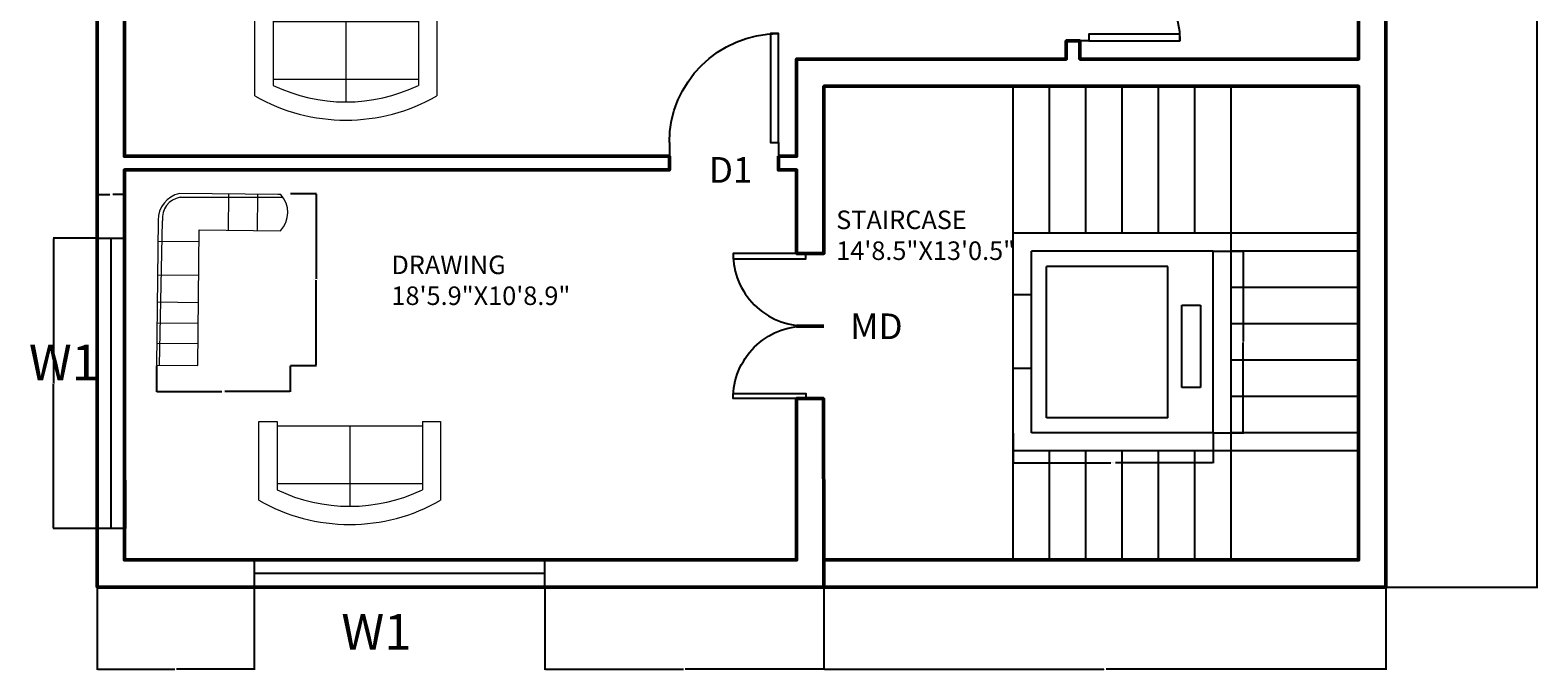
# Model space of a CAD drawing. Units: inches. Extents: x -45 to 1424, y 648 to 1662.
# Tile 5 of 8: x 927 to 1424, y 695 to 906. Entities that reach past the tile are written whole.
import ezdxf

# ---------------------------------------------------------------- set-up
doc = ezdxf.new("R2010")
doc.units = ezdxf.units.IN
for name, color, linetype, lineweight in [('A-ANNO-DIMS', 2, 'Continuous', 18), ('A-ANNO-TEXT', 7, 'Continuous', 18), ('A-AREA-IDEN', 7, 'Continuous', 18), ('A-FLOR-EVTR', 140, 'Continuous', 25), ('DOOR', 2, 'Continuous', 25), ('FURNITURE', 3, 'Continuous', 18), ('STAIRCASE', 140, 'Continuous', 25), ('WALL', 4, 'Continuous', 50), ('WINDOW', 1, 'Continuous', 25)]:
    doc.layers.add(name, color=color, linetype=linetype, lineweight=lineweight)
doc.styles.get("Standard").update_dxf_attribs({"font": 'arial.ttf'})
doc.dimstyles.get("Standard").update_dxf_attribs({"dimtxt": 0.18, "dimasz": 0.18, "dimexe": 0.18, "dimexo": 0.0625, "dimgap": 0.09, "dimtad": 0, "dimtih": 1, "dimtoh": 1, "dimdec": 4, "dimzin": 0, "dimdsep": 46, "dimtxsty": 'Standard', "dimcen": 0.09, "dimadec": 0, "dimazin": 0, "dimtfac": 1, "dimtdec": 4, "dimtofl": 0, "dimtmove": 0, "dimatfit": 3, "dimfxl": 1, "dimtolj": 1, "dimtzin": 0, "dimarcsym": 0})

# ---------------------------------------------------------------- blocks, each defined once
blk = doc.blocks.new('*U5')
for p, q in [((0, 0), (0, -6)), ((24, 0), (24, -6))]:
    blk.add_line(p, q)
blk.add_lwpolyline([(0, 0), (0, 24), (1.75, 24), (1.75, 0)], close=True)
blk.add_arc((0, 0), 24, 0, 90)
blk = doc.blocks.new('*U3')
for p, q in [((0, 0), (0, -6)), ((24, 0), (24, -6))]:
    blk.add_line(p, q)
blk.add_lwpolyline([(0, 0), (0, 24), (1.75, 24), (1.75, 0)], close=True)
blk.add_arc((0, 0), 24, 0, 90)
blk = doc.blocks.new('*U6')
for p, q in [((0, 0), (0, 6)), ((24, 0), (24, 6))]:
    blk.add_line(p, q)
blk.add_lwpolyline([(0, 0), (0, -24), (1.75, -24), (1.75, 0)], close=True)
blk.add_arc((0, 0), 24, 270, 0)
blk = doc.blocks.new('Sofa - Roundback Loveseat 5 ft.')
for p, q in [((0, -32.44198), (0, -5.99998)), ((-24, -33.99998), (-24, -11.46958)), ((-23.9998, -13.38178), (23.99986, -13.38178)), ((24.00004, -33.99998), (24.00004, -11.46958)), ((-24, -32.44198), (24.00004, -32.44198))]:
    blk.add_line(p, q)
for points in [[(-24, -33.99998), (-30, -33.99998), (-30, -7.99998)], [(30.00004, -7.99998), (30.00004, -33.99998), (24.00004, -33.99998)]]:
    blk.add_lwpolyline(points)
for centre, radius, start, end in [((0, -60.24998), 60.24998, 60.13715, 119.8628), ((0, -61.38438), 55.38444, 64.32083, 115.6792)]:
    blk.add_arc(centre, radius, start, end)
blk = doc.blocks.new('WIN-W1-DRAWING-W')
for p, q in [((0, 96), (9, 96)), ((0, 0), (0, 96)), ((4.66, 0), (4.66, 96)), ((9, 96), (9.31, 0)), ((9.31, 0), (0, 0))]:
    blk.add_line(p, q)
blk = doc.blocks.new('WIN-W1-DRAWING-S')
for p, q in [((0, 9), (0, 0)), ((96, 9), (0, 9)), ((96, 0.07), (96, 9)), ((96, 4.53), (0, 4.53)), ((0, 0), (96, 0.07))]:
    blk.add_line(p, q)
blk = doc.blocks.new('FURN-CORNER-UNIT')
for p, q in [((40.07, 56.49), (7.6, 56.85)), ((7.84, 55.59), (41.8, 55.6)), ((23.84, 56.67), (23.71, 44.7)), ((33.42, 56.57), (33.29, 44.59)), ((41.09, 56.48), (40.07, 56.49)), ((0.52, 47.99), (0, 0.15)), ((1.05, 0.14), (1.97, 47.86)), ((13.64, 0), (14.13, 44.8)), ((14.13, 44.8), (40.96, 44.51)), ((14.09, 40.87), (0.45, 41.02)), ((13.96, 29.74), (0.33, 29.89)), ((13.86, 20.75), (0.23, 20.9)), ((13.79, 13.89), (0.15, 14.04)), ((13.72, 7.15), (0.08, 7.29)), ((0, 0.15), (13.64, 0))]:
    blk.add_line(p, q)
for centre, radius, start, end in [((9.61, 47.99), 9.08, 102.7689, 180), ((8.93, 48.68), 7, 98.9855, 186.697), ((34.55, 50.57), 8.82, 316.6036, 42.1383)]:
    blk.add_arc(centre, radius, start, end)
blk = doc.blocks.new('STAIR-RETURN')
for p, q in [((0, 0), (0, 156.5)), ((12, 108), (12, 156.5)), ((24, 108), (24, 156.5)), ((36, 108), (36, 156.5)), ((48, 108), (48, 156.5)), ((60, 108), (60, 156.5)), ((72, 0), (72, 156.5)), ((114, 108), (0, 108)), ((114, 102), (72, 102)), ((114, 90), (72, 90)), ((114, 78), (72, 78)), ((114, 66), (72, 66)), ((114, 66), (72, 66)), ((114, 66), (72, 66)), ((114, 66), (72, 66)), ((114, 54), (72, 54)), ((114, 42), (72, 42)), ((114, 36), (0, 36)), ((12, 0), (12, 36)), ((24, 0), (24, 36)), ((36, 0), (36, 36)), ((48, 0), (48, 36)), ((60, 0), (60, 36))]:
    blk.add_line(p, q)
blk = doc.blocks.new('LIFT-PLAN')
for p, q in [((6, 0), (6, 60)), ((66, 60), (6, 60)), ((66, 0), (66, 60)), ((11, 5), (11, 55)), ((51, 55), (11, 55)), ((51, 5), (51, 55)), ((0, 45.73), (6, 45.73)), ((55.71, 14.94), (55.71, 42.13)), ((55.71, 42.13), (61.81, 42.13)), ((61.81, 42.13), (61.81, 14.94)), ((0, 21.36), (6, 21.36)), ((61.81, 14.94), (55.71, 14.94)), ((51, 5), (11, 5)), ((66, 0), (6, 0))]:
    blk.add_line(p, q)
blk = doc.blocks.new('*D62')
at = {"layer": 'A-ANNO-DIMS', "color": 0, "lineweight": -2, "transparency": 16777216}
for p, q in [((948.79, 837.18), (934.27, 837.18)), ((934.45, 837), (934.45, 789.36)), ((934.45, 741.36), (934.45, 789)), ((948.79, 741.18), (934.27, 741.18))]:
    blk.add_line(p, q, dxfattribs=at)
at = {"layer": 'A-ANNO-DIMS', "color": 0, "transparency": 16777216}
for points in [[(934.42, 837), (934.48, 837), (934.45, 837.18)], [(934.42, 741.36), (934.48, 741.36), (934.45, 741.18)]]:
    blk.add_solid(points, dxfattribs=at)
at = {"layer": 'Defpoints', "color": 0, "transparency": 16777216}
for p in [(934.45, 837.18), (948.85, 837.18), (948.85, 741.18)]:
    blk.add_point(p, dxfattribs=at)
at = {"layer": 'A-ANNO-DIMS', "color": 0, "transparency": 16777216, "insert": (934.45, 789.18), "char_height": 0.18, "attachment_point": 5}
blk.add_mtext('\\A1;W1 96 TYP.', dxfattribs=at)
blk = doc.blocks.new('*D63')
at = {"layer": 'A-ANNO-DIMS', "color": 0, "lineweight": -2, "transparency": 16777216}
for p, q in [((948.85, 837.24), (948.85, 851.76)), ((949.03, 851.58), (953.05, 851.58)), ((957.99, 851.58), (953.97, 851.58)), ((958.17, 837.24), (958.17, 851.76))]:
    blk.add_line(p, q, dxfattribs=at)
at = {"layer": 'A-ANNO-DIMS', "color": 0, "transparency": 16777216}
for points in [[(949.03, 851.61), (949.03, 851.55), (948.85, 851.58)], [(957.99, 851.61), (957.99, 851.55), (958.17, 851.58)]]:
    blk.add_solid(points, dxfattribs=at)
at = {"layer": 'Defpoints', "color": 0, "transparency": 16777216}
for p in [(958.17, 851.58), (948.85, 837.18), (958.17, 837.18)]:
    blk.add_point(p, dxfattribs=at)
at = {"layer": 'A-ANNO-DIMS', "color": 0, "transparency": 16777216, "insert": (953.51, 851.58), "char_height": 0.18, "attachment_point": 5}
blk.add_mtext('\\A1;9 TYP.', dxfattribs=at)
blk = doc.blocks.new('*D66')
at = {"layer": 'A-ANNO-DIMS', "color": 0, "lineweight": -2, "transparency": 16777216}
for p, q in [((1012.65, 851.93), (1021.3, 851.93)), ((1021.12, 851.75), (1021.12, 823.69)), ((1021.12, 795.26), (1021.12, 823.32)), ((1012.65, 795.08), (1021.3, 795.08))]:
    blk.add_line(p, q, dxfattribs=at)
at = {"layer": 'A-ANNO-DIMS', "color": 0, "transparency": 16777216}
for points in [[(1021.09, 851.75), (1021.15, 851.75), (1021.12, 851.93)], [(1021.09, 795.26), (1021.15, 795.26), (1021.12, 795.08)]]:
    blk.add_solid(points, dxfattribs=at)
at = {"layer": 'Defpoints', "color": 0, "transparency": 16777216}
for p in [(1012.59, 851.93), (1021.12, 851.93), (1012.59, 795.08)]:
    blk.add_point(p, dxfattribs=at)
at = {"layer": 'A-ANNO-DIMS', "color": 0, "transparency": 16777216, "insert": (1021.12, 823.5), "char_height": 0.18, "attachment_point": 5}
blk.add_mtext('\\A1;CORNER UNIT 57 TYP.', dxfattribs=at)
blk = doc.blocks.new('*D67')
at = {"layer": 'A-ANNO-DIMS', "color": 0, "lineweight": -2, "transparency": 16777216}
for p, q in [((968.41, 795.02), (968.41, 786.37)), ((1012.59, 795.02), (1012.59, 786.37)), ((968.59, 786.55), (989.97, 786.55)), ((1012.41, 786.55), (991.03, 786.55))]:
    blk.add_line(p, q, dxfattribs=at)
at = {"layer": 'A-ANNO-DIMS', "color": 0, "transparency": 16777216}
for points in [[(968.59, 786.58), (968.59, 786.52), (968.41, 786.55)], [(1012.41, 786.58), (1012.41, 786.52), (1012.59, 786.55)]]:
    blk.add_solid(points, dxfattribs=at)
at = {"layer": 'Defpoints', "color": 0, "transparency": 16777216}
for p in [(968.41, 795.08), (1012.59, 795.08), (1012.59, 786.55)]:
    blk.add_point(p, dxfattribs=at)
at = {"layer": 'A-ANNO-DIMS', "color": 0, "transparency": 16777216, "insert": (990.5, 786.55), "char_height": 0.18, "attachment_point": 5}
blk.add_mtext('\\A1;44 TYP.', dxfattribs=at)
blk = doc.blocks.new('*D72')
at = {"layer": 'A-ANNO-DIMS', "color": 0, "lineweight": -2, "transparency": 16777216}
for p, q in [((1251.25, 772.78), (1251.25, 762.77)), ((1317.25, 772.78), (1317.25, 762.77)), ((1251.43, 762.95), (1283.44, 762.95)), ((1317.07, 762.95), (1285.07, 762.95))]:
    blk.add_line(p, q, dxfattribs=at)
at = {"layer": 'A-ANNO-DIMS', "color": 0, "transparency": 16777216}
for points in [[(1251.43, 762.98), (1251.43, 762.92), (1251.25, 762.95)], [(1317.07, 762.98), (1317.07, 762.92), (1317.25, 762.95)]]:
    blk.add_solid(points, dxfattribs=at)
at = {"layer": 'Defpoints', "color": 0, "transparency": 16777216}
for p in [(1251.25, 772.85), (1317.25, 772.85), (1317.25, 762.95)]:
    blk.add_point(p, dxfattribs=at)
at = {"layer": 'A-ANNO-DIMS', "color": 0, "transparency": 16777216, "insert": (1284.25, 762.95), "char_height": 0.18, "attachment_point": 5}
blk.add_mtext('\\A1;LIFT 66 TYP.', dxfattribs=at)
blk = doc.blocks.new('*D73')
at = {"layer": 'A-ANNO-DIMS', "color": 0, "lineweight": -2, "transparency": 16777216}
for p, q in [((1317.32, 832.85), (1327.33, 832.85)), ((1327.15, 832.67), (1327.15, 803.03)), ((1327.15, 773.03), (1327.15, 802.66)), ((1317.32, 772.85), (1327.33, 772.85))]:
    blk.add_line(p, q, dxfattribs=at)
at = {"layer": 'A-ANNO-DIMS', "color": 0, "transparency": 16777216}
for points in [[(1327.12, 832.67), (1327.18, 832.67), (1327.15, 832.85)], [(1327.12, 773.03), (1327.18, 773.03), (1327.15, 772.85)]]:
    blk.add_solid(points, dxfattribs=at)
at = {"layer": 'Defpoints', "color": 0, "transparency": 16777216}
for p in [(1317.25, 832.85), (1327.15, 832.85), (1317.25, 772.85)]:
    blk.add_point(p, dxfattribs=at)
at = {"layer": 'A-ANNO-DIMS', "color": 0, "transparency": 16777216, "insert": (1327.15, 802.85), "char_height": 0.18, "attachment_point": 5}
blk.add_mtext('\\A1;60 TYP.', dxfattribs=at)
blk = doc.blocks.new('*D83')
at = {"layer": 'A-ANNO-DIMS', "color": 0, "lineweight": -2, "transparency": 16777216}
for p, q in [((1374.32, 1189.85), (1424.39, 1189.85)), ((1424.21, 1189.67), (1424.21, 956.03)), ((1424.21, 722.03), (1424.21, 955.67)), ((1374.32, 721.85), (1424.39, 721.85))]:
    blk.add_line(p, q, dxfattribs=at)
at = {"layer": 'A-ANNO-DIMS', "color": 0, "transparency": 16777216}
for points in [[(1424.18, 1189.67), (1424.24, 1189.67), (1424.21, 1189.85)], [(1424.18, 722.03), (1424.24, 722.03), (1424.21, 721.85)]]:
    blk.add_solid(points, dxfattribs=at)
at = {"layer": 'Defpoints', "color": 0, "transparency": 16777216}
for p in [(1374.25, 1189.85), (1424.21, 1189.85), (1374.25, 721.85)]:
    blk.add_point(p, dxfattribs=at)
at = {"layer": 'A-ANNO-DIMS', "color": 0, "transparency": 16777216, "insert": (1424.21, 955.85), "char_height": 0.18, "attachment_point": 5}
blk.add_mtext('\\A1;468', dxfattribs=at)
blk = doc.blocks.new('*D84')
at = {"layer": 'A-ANNO-DIMS', "color": 0, "lineweight": -2, "transparency": 16777216}
for p, q in [((948.85, 721.79), (948.85, 694.52)), ((1000.65, 721.79), (1000.65, 694.52)), ((949.03, 694.7), (974.43, 694.7)), ((1000.47, 694.7), (975.08, 694.7))]:
    blk.add_line(p, q, dxfattribs=at)
at = {"layer": 'A-ANNO-DIMS', "color": 0, "transparency": 16777216}
for points in [[(949.03, 694.73), (949.03, 694.67), (948.85, 694.7)], [(1000.47, 694.73), (1000.47, 694.67), (1000.65, 694.7)]]:
    blk.add_solid(points, dxfattribs=at)
at = {"layer": 'Defpoints', "color": 0, "transparency": 16777216}
for p in [(948.85, 721.85), (1000.65, 721.85), (1000.65, 694.7)]:
    blk.add_point(p, dxfattribs=at)
at = {"layer": 'A-ANNO-DIMS', "color": 0, "transparency": 16777216, "insert": (974.75, 694.7), "char_height": 0.18, "attachment_point": 5}
blk.add_mtext('\\A1;51.8', dxfattribs=at)
blk = doc.blocks.new('*D85')
at = {"layer": 'A-ANNO-DIMS', "color": 0, "lineweight": -2, "transparency": 16777216}
for p, q in [((1096.65, 721.85), (1096.65, 694.52)), ((1188.75, 721.79), (1188.75, 694.52)), ((1096.83, 694.7), (1142.4, 694.7)), ((1188.57, 694.7), (1143.01, 694.7))]:
    blk.add_line(p, q, dxfattribs=at)
at = {"layer": 'A-ANNO-DIMS', "color": 0, "transparency": 16777216}
for points in [[(1096.83, 694.73), (1096.83, 694.67), (1096.65, 694.7)], [(1188.57, 694.73), (1188.57, 694.67), (1188.75, 694.7)]]:
    blk.add_solid(points, dxfattribs=at)
at = {"layer": 'Defpoints', "color": 0, "transparency": 16777216}
for p in [(1096.65, 721.92), (1188.75, 721.85), (1188.75, 694.7)]:
    blk.add_point(p, dxfattribs=at)
at = {"layer": 'A-ANNO-DIMS', "color": 0, "transparency": 16777216, "insert": (1142.7, 694.7), "char_height": 0.18, "attachment_point": 5}
blk.add_mtext('\\A1;92.1', dxfattribs=at)
blk = doc.blocks.new('*D86')
at = {"layer": 'A-ANNO-DIMS', "color": 0, "lineweight": -2, "transparency": 16777216}
for p, q in [((1188.75, 721.79), (1188.75, 694.52)), ((1374.25, 721.79), (1374.25, 694.52)), ((1188.93, 694.7), (1281.12, 694.7)), ((1374.07, 694.7), (1281.89, 694.7))]:
    blk.add_line(p, q, dxfattribs=at)
at = {"layer": 'A-ANNO-DIMS', "color": 0, "transparency": 16777216}
for points in [[(1188.93, 694.73), (1188.93, 694.67), (1188.75, 694.7)], [(1374.07, 694.73), (1374.07, 694.67), (1374.25, 694.7)]]:
    blk.add_solid(points, dxfattribs=at)
at = {"layer": 'Defpoints', "color": 0, "transparency": 16777216}
for p in [(1188.75, 721.85), (1374.25, 721.85), (1374.25, 694.7)]:
    blk.add_point(p, dxfattribs=at)
at = {"layer": 'A-ANNO-DIMS', "color": 0, "transparency": 16777216, "insert": (1281.5, 694.7), "char_height": 0.18, "attachment_point": 5}
blk.add_mtext('\\A1;185.5', dxfattribs=at)

msp = doc.modelspace()

# ---------------------------------------------------------------- linework, layer by layer
at = {"layer": 'WALL'}
msp.add_line((1188.7541, 808.1394), (1179.7541, 808.1394), dxfattribs=at)
msp.add_lwpolyline([(1374.2541, 1189.8478), (1374.2541, 721.8478), (948.8541, 721.8478), (948.8541, 1189.8478)], close=True, dxfattribs=at)
for points in [[(1188.7541, 721.8478), (1188.7541, 730.8478), (1188.5825, 784.14), (1179.7541, 784.14), (1179.7541, 730.8478), (957.8541, 730.8478), (957.8541, 859.7478), (1137.7546, 859.7478), (1137.7546, 864.2478), (957.8541, 864.2478), (957.8541, 1033.8478), (1052.8542, 1033.8478)], [(1279.2525, 896.3478), (1365.2541, 896.3478), (1365.2541, 948.8478), (1273.2541, 948.8478), (1273.2541, 932.34), (1268.7541, 932.34), (1268.7541, 1011.3478), (1266.755, 1011.3478)], [(1279.2525, 896.3478), (1273.2541, 896.3478), (1273.2541, 902.3401), (1268.7541, 902.3401), (1268.7541, 896.3478), (1179.7541, 896.3478), (1179.7541, 864.2478), (1173.7545, 864.2478)], [(1188.7541, 832.1388), (1188.7541, 887.3478), (1188.7541, 832.1388), (1179.7541, 832.1388), (1179.7541, 859.7478), (1173.7545, 859.7478), (1173.7545, 864.2478)], [(1188.7541, 887.3478), (1365.2541, 887.3478), (1365.2541, 730.8478), (1188.7541, 730.8478)]]:
    msp.add_lwpolyline(points, dxfattribs=at)

# ---------------------------------------------------------------- block references
at = {"layer": 'A-FLOR-EVTR'}
msp.add_blockref('LIFT-PLAN', (1251.2541, 772.8468), dxfattribs=at)
at = {"layer": 'DOOR', "xscale": -1.25, "yscale": 1.25, "zscale": 1.25, "rotation": 270}
msp.add_blockref('*U5', (1276.2541, 902.3401), dxfattribs=at)
at = {"layer": 'DOOR', "xscale": -1.5, "yscale": 1.5, "zscale": 1.5}
msp.add_blockref('*U3', (1173.7545, 868.7478), dxfattribs=at)
at = {"layer": 'DOOR', "rotation": 270}
msp.add_blockref('*U6', (1182.7541, 832.1394), dxfattribs=at)
at = {"layer": 'DOOR', "xscale": -1, "rotation": 270}
msp.add_blockref('*U6', (1182.7541, 784.1394), dxfattribs=at)
at = {"layer": 'FURNITURE', "rotation": 180}
for p in [(1030.9343, 876.1746), (1032.2201, 742.5611)]:
    msp.add_blockref('Sofa - Roundback Loveseat 5 ft.', p, dxfattribs=at)
at = {"layer": 'FURNITURE'}
msp.add_blockref('FURN-CORNER-UNIT', (968.4081, 795.0798), dxfattribs=at)
at = {"layer": 'STAIRCASE'}
msp.add_blockref('STAIR-RETURN', (1251.2541, 730.8478), dxfattribs=at)
at = {"layer": 'WINDOW'}
for name, p in [('WIN-W1-DRAWING-W', (948.8541, 741.1788)), ('WIN-W1-DRAWING-S', (1000.6501, 721.8478))]:
    msp.add_blockref(name, p, dxfattribs=at)

# ---------------------------------------------------------------- texts
at = {"layer": 'A-ANNO-TEXT', "attachment_point": 1}
for s, width, gutter_width, insert, char_height in [('D1', 8.475535, 42.3777, (1150.7828, 863.9706), 8.47554), ('MD', 8.475535, 42.3777, (1197.3981, 812.2817), 8.47554), ('W1', 18.68524, 59.1031, (926.3038, 802.0061), 11.82062), ('W1', 18.68524, 59.1031, (1029.4528, 712.967), 11.82062)]:
    msp.add_mtext_dynamic_manual_height_columns(s, width=width, gutter_width=gutter_width, heights=[0], dxfattribs=dict(at, insert=insert, char_height=char_height))
at = {"layer": 'A-AREA-IDEN', "char_height": 6.122202, "attachment_point": 1}
for s, insert in [('STAIRCASE\\P14\'8.5"X13\'0.5"', (1192.8171, 846.291)), ('DRAWING\\P18\'5.9"X10\'8.9"', (1045.9863, 831.4124))]:
    msp.add_mtext(s, dxfattribs=dict(at, insert=insert))

# ---------------------------------------------------------------- dimensions: what is measured, and where the dimension line sits
at = {"layer": 'A-ANNO-DIMS'}
dim = msp.add_linear_dim(base=(1424.2072, 1189.8478), p1=(1374.2541, 721.8478), p2=(1374.2541, 1189.8478), angle=90, dimstyle='Standard', override={"dimdec": 0, "dimlfac": 1, "dimrnd": 0, "dimzin": 0, "dimdsep": 46, "dimlunit": 2}, dxfattribs=at)
dim.commit()
dim.dimension.update_dxf_attribs({"geometry": '*D83', "text_midpoint": (1424.2072, 955.8478)})
for base, p1, p2, text, picture, middle in [((958.1679, 851.5779), (948.8541, 837.178), (958.1679, 837.178), '<> TYP.', '*D63', (953.511, 851.5779)), ((1012.5908, 786.5521), (968.4078, 795.0796), (1012.5908, 795.0796), '<> TYP.', '*D67', (990.4993, 786.5521)), ((1317.2541, 762.9467), (1251.2541, 772.8467), (1317.2541, 772.8467), 'LIFT <> TYP.', '*D72', (1284.2541, 762.9467))]:
    dim = msp.add_linear_dim(base=base, p1=p1, p2=p2, text=text, dimstyle='Standard', override={"dimdec": 0, "dimlfac": 1, "dimrnd": 0, "dimzin": 0, "dimdsep": 46, "dimlunit": 2}, dxfattribs=at)
    dim.commit()
    dim.dimension.update_dxf_attribs({"geometry": picture, "text_midpoint": middle})
for base, p1, p2, text, picture, middle in [((1021.1183, 851.93), (1012.5908, 795.0796), (1012.5908, 851.93), 'CORNER UNIT <> TYP.', '*D66', (1021.1183, 823.5048)), ((934.4542, 837.178), (948.8541, 741.1785), (948.8541, 837.178), 'W1 <> TYP.', '*D62', (934.4542, 789.1783)), ((1327.1541, 832.8467), (1317.2541, 772.8467), (1317.2541, 832.8467), '<> TYP.', '*D73', (1327.1541, 802.8467))]:
    dim = msp.add_linear_dim(base=base, p1=p1, p2=p2, angle=90, text=text, dimstyle='Standard', override={"dimdec": 0, "dimlfac": 1, "dimrnd": 0, "dimzin": 0, "dimdsep": 46, "dimlunit": 2}, dxfattribs=at)
    dim.commit()
    dim.dimension.update_dxf_attribs({"geometry": picture, "text_midpoint": middle})
for base, p1, p2, picture, middle in [((1000.6502, 694.6978), (948.8541, 721.8478), (1000.6502, 721.8478), '*D84', (974.7522, 694.6978)), ((1188.7541, 694.6978), (1096.6502, 721.9156), (1188.7541, 721.8478), '*D85', (1142.7022, 694.6978)), ((1374.2541, 694.6978), (1188.7541, 721.8478), (1374.2541, 721.8478), '*D86', (1281.5041, 694.6978))]:
    dim = msp.add_linear_dim(base=base, p1=p1, p2=p2, dimstyle='Standard', override={"dimdec": 1, "dimlfac": 1, "dimrnd": 0, "dimzin": 0, "dimdsep": 46, "dimlunit": 2}, dxfattribs=at)
    dim.commit()
    dim.dimension.update_dxf_attribs({"geometry": picture, "text_midpoint": middle})

doc.saveas('drawing.dxf')
